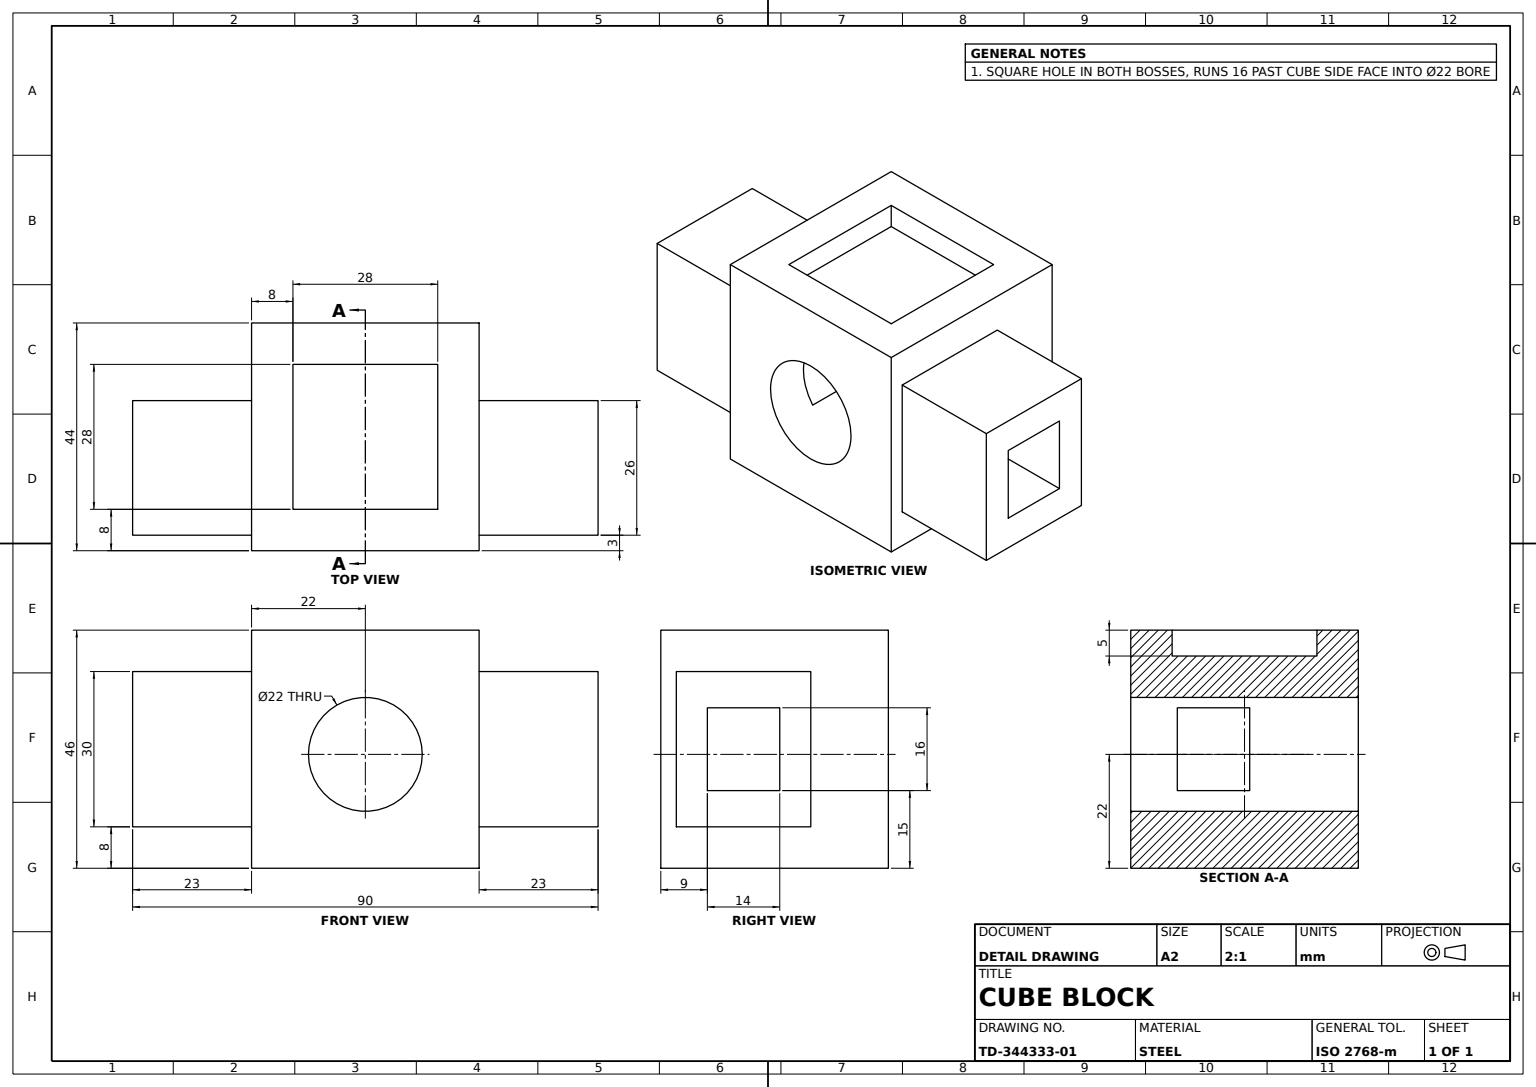
from build123d import *

# Parameters (mm, degrees)
MAIN_BLOCK_PROFILE_W            = 44
MAIN_BLOCK_PROFILE_H            = 46
MAIN_BLOCK_PROFILE_R            = 11
MAIN_BLOCK_44MM_DEPTH           = 44
TOP_POCKET_PROFILE_28X28_W      = 28
TOP_POCKET_PROFILE_28X28_H      = 28
TOP_SQUARE_POCKET_28X28X5_DEPTH = 5
SIDE_BOSS_PROFILE_W             = 26
SIDE_BOSS_PROFILE_H             = 30
SIDE_BOSS_PROFILE_W_2           = 14
SIDE_BOSS_PROFILE_H_2           = 16
SIDE_SQUARE_BOSS_23MM_DEPTH     = 23
SIDE_OPENING_PROFILE_W          = 14
SIDE_OPENING_PROFILE_H          = 16
SIDE_OPENING_CUT_DEPTH          = 103.786185842


with BuildPart() as part:
    # Main Block Profile → Main Block 44mm (new body)
    with BuildSketch(Plane.XY):
        Rectangle(MAIN_BLOCK_PROFILE_W, MAIN_BLOCK_PROFILE_H)
        with Locations((0, -1)):
            Circle(MAIN_BLOCK_PROFILE_R, mode=Mode.SUBTRACT)
    extrude(amount=-MAIN_BLOCK_44MM_DEPTH)

    # Top Pocket Profile 28x28 → Top Square Pocket 28x28x5 (cut)
    with BuildSketch(Plane(origin=(0, 23, 0), x_dir=(1, 0, 0), z_dir=(0, 1, 0))):
        with Locations((0, 22)):
            Rectangle(TOP_POCKET_PROFILE_28X28_W, TOP_POCKET_PROFILE_28X28_H)
    extrude(amount=-TOP_SQUARE_POCKET_28X28X5_DEPTH, mode=Mode.SUBTRACT)

    # Side Boss Profile → Side Square Boss 23mm (add)
    with BuildSketch(Plane.ZY.offset(22)):
        with Locations((-16, 0)):
            Rectangle(SIDE_BOSS_PROFILE_W, SIDE_BOSS_PROFILE_H)
        with Locations((-16, 0)):
            Rectangle(SIDE_BOSS_PROFILE_W_2, SIDE_BOSS_PROFILE_H_2, mode=Mode.SUBTRACT)
    side_square_boss_23mm = extrude(amount=SIDE_SQUARE_BOSS_23MM_DEPTH)

    # Side Boss Mirror: Side Square Boss 23mm across plane
    add(side_square_boss_23mm.mirror(Plane(origin=(0, 0, 0), x_dir=(0, 0, 1), z_dir=(1, 0, 0))))

    # Side Opening Profile → Side Opening Cut (cut, through all)
    with BuildSketch(Plane(origin=(45, 0, 0), x_dir=(0, 0, -1), z_dir=(1, 0, 0))):
        with Locations((16, 0)):
            Rectangle(SIDE_OPENING_PROFILE_W, SIDE_OPENING_PROFILE_H)
    extrude(amount=-SIDE_OPENING_CUT_DEPTH, mode=Mode.SUBTRACT)


solid = part.part
